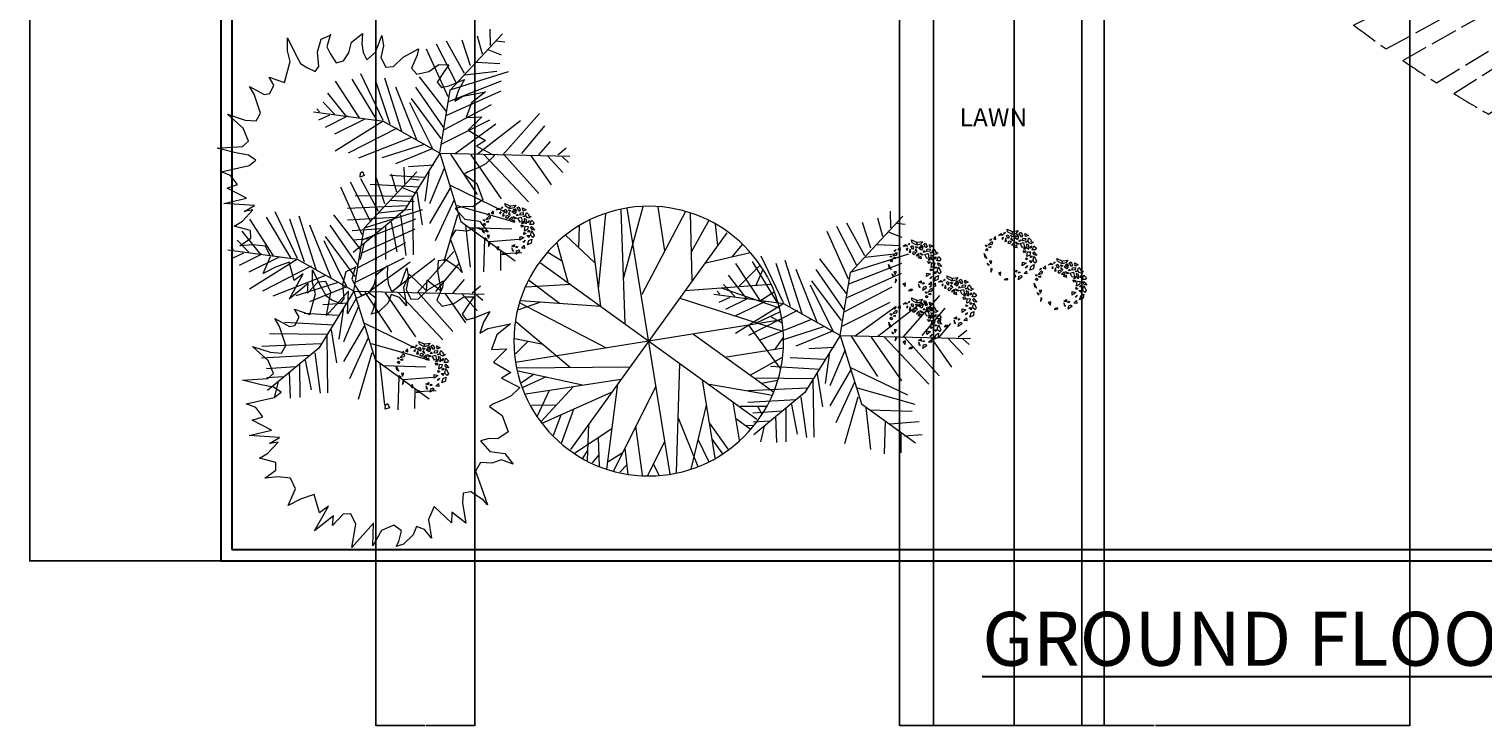
# Model space of a CAD drawing. Units: inches. Extents: x 2330 to 3943, y 1763 to 3461.
# Tile 1 of 40: x 2330 to 2977, y 1901 to 2211. Entities that reach past the tile are written whole.
import ezdxf

# ---------------------------------------------------------------- set-up
doc = ezdxf.new("R2010")
doc.units = ezdxf.units.IN
doc.linetypes.add('ACAD_ISO02W100', pattern=[15, 12, -3])
for name, color, linetype, lineweight in [('A-ANNO-DIMS', 2, 'Continuous', 18), ('A-ANNO-TEXT', 7, 'Continuous', 18), ('A-ANNO-TITL', 7, 'Continuous', 30), ('C-PROP', 7, 'Continuous', 30), ('L-PLNT', 94, 'Continuous', 13), ('L-PVMT-JOIN', 9, 'ACAD_ISO02W100', 13)]:
    doc.layers.add(name, color=color, linetype=linetype, lineweight=lineweight)
doc.styles.get("Standard").update_dxf_attribs({"font": 'arial.ttf'})
doc.dimstyles.get("Standard").update_dxf_attribs({"dimtxt": 0.18, "dimasz": 0.18, "dimexe": 0.18, "dimexo": 0.0625, "dimgap": 0.09, "dimtad": 0, "dimtih": 1, "dimtoh": 1, "dimdec": 4, "dimzin": 0, "dimdsep": 46, "dimtxsty": 'Standard', "dimcen": 0.09, "dimadec": 0, "dimazin": 0, "dimtfac": 1, "dimtdec": 4, "dimtofl": 0, "dimtmove": 0, "dimatfit": 3, "dimfxl": 1, "dimtolj": 1, "dimtzin": 0, "dimarcsym": 0})

# ---------------------------------------------------------------- blocks, each defined once
blk = doc.blocks.new('*U12')
for p, q in [((-8.737, 47.138), (-17.069, 52.711)), ((-10.186, 53.64), (-13.084, 55.962)), ((0, 0), (-10.5, 57)), ((-9.099, 51.782), (-6.563, 55.962)), ((-7.288, 39.707), (-21.778, 46.673)), ((-7.65, 43.423), (-2.578, 49.46)), ((-5.839, 35.992), (4.667, 48.067)), ((-5.114, 27.632), (10.463, 46.673)), ((-5.114, 28.097), (-24.676, 40.636)), ((-3.665, 19.273), (-27.574, 35.527)), ((-2.941, 16.486), (8.652, 37.85)), ((27, 9), (48, 36)), ((27.127, 9.056), (31.112, 35.992)), ((35.096, 32.741), (37.27, 22.524)), ((38.719, 34.134), (41.979, 28.561)), ((44.153, 36.456), (45.239, 32.741)), ((-48.585, 21.131), (-49.309, 29.026)), ((-43.513, 28.561), (-42.427, 15.558)), ((-38.442, 26.239), (-34.819, 7.663)), ((-35.544, 28.097), (-24.314, 3.947)), ((-1.129, 6.734), (9.014, 26.704)), ((10.101, 3.483), (17.708, 26.239)), ((16.259, 5.805), (23.142, 31.348)), ((22.055, 7.198), (27.489, 32.277)), ((31.836, 30.883), (32.561, 16.486)), ((43.791, 29.954), (51.036, 30.883)), ((-47.498, 19.737), (-55.83, 18.344)), ((-31.5, 4.5), (-52.5, 25.5)), ((-14.533, 2.09), (-30.834, 25.31)), ((-24.314, 23.917), (-2.941, 13.7)), ((3.942, 1.625), (11.187, 24.381)), ((36.183, 19.737), (48.137, 17.88)), ((40.53, 25.775), (48.862, 24.846)), ((-40.615, 13.7), (-55.105, 10.913)), ((-20.691, 13.7), (-1.129, 4.876)), ((33.285, 16.486), (48.862, 10.913)), ((0, 0), (27, 9)), ((24.229, 7.663), (46.688, 1.625)), ((29.662, 12.307), (48.137, 6.269)), ((-33.37, 6.269), (-52.207, 5.34)), ((-28.299, 3.483), (-47.86, -5.805)), ((-21.416, 3.018), (-38.079, -8.128)), ((0, 0), (-31.5, 4.5)), ((-15.982, 2.09), (-30.11, -9.521)), ((0, 0), (-22.5, -19.5)), ((-6.563, 1.161), (-21.416, -8.128)), ((0, 0), (18, -22.5)), ((6.478, 1.625), (26.04, -8.592)), ((11.187, 3.483), (30.749, -5.805)), ((18.07, 5.805), (35.096, -3.483)), ((-6.563, -5.805), (-19.967, -9.985)), ((-4.752, -3.483), (-3.665, -14.629)), ((2.493, -3.019), (-1.491, -20.202)), ((1.769, -2.555), (24.229, -9.521)), ((5.029, -6.27), (2.131, -25.775)), ((-15.257, -12.772), (-30.11, -12.772)), ((-13.446, -11.378), (-8.737, -32.741)), ((-9.461, -8.592), (-6.201, -23.453)), ((9.014, -11.378), (3.58, -35.992)), ((7.565, -9.056), (32.198, -14.629)), ((-17.431, -15.094), (-42.789, -18.809)), ((-20.691, -18.345), (-17.793, -44.352)), ((-17.069, -15.094), (-12.721, -40.172)), ((14.085, -16.951), (6.478, -40.172)), ((12.274, -15.094), (36.907, -18.809)), ((-24.314, -21.596), (-42.427, -22.06)), ((-26.849, -26.24), (-40.253, -25.775)), ((-22.5, -19.5), (-37.5, -45)), ((-25.038, -23.918), (-22.865, -45.281)), ((18.07, -22.524), (8.289, -45.745)), ((16.259, -19.738), (36.183, -22.989)), ((18, -22.5), (27, -52.5)), ((18.433, -22.524), (40.53, -29.026)), ((19.157, -25.311), (38.719, -33.206)), ((-28.299, -29.026), (-42.789, -31.348)), ((-29.023, -30.884), (-27.936, -43.887)), ((20.244, -30.419), (15.897, -44.816)), ((-30.834, -34.135), (-42.427, -35.528)), ((-32.646, -36.921), (-31.921, -44.352)), ((22.78, -37.85), (19.519, -48.532)), ((21.331, -32.741), (39.081, -40.636)), ((22.78, -38.314), (34.372, -44.816)), ((-34.457, -39.708), (-40.978, -42.494)), ((24.591, -43.423), (30.749, -47.603)), ((24.591, -45.745), (23.142, -50.854)), ((26.764, -49.925), (28.213, -50.854))]:
    blk.add_line(p, q)
blk = doc.blocks.new('*U13')
for points in [[(-5.78, 9.75), (-7.54, 9.23), (-8.01, 7.5), (-6.26, 8.45)], [(-5.78, 6.81), (-6.66, 6.21), (-6.52, 5.69)], [(-4.43, 11.05), (-5.18, 10.36), (-3.96, 9.49), (-2.07, 10.36)], [(-4.84, 8.63), (-3.83, 7.85), (-4.03, 8.97)], [(-2.88, 7.5), (-3.15, 6.64), (-2.27, 6.72)], [(-1.94, 9.49), (-2.48, 8.97), (-2.27, 8.54), (-1.8, 9.06)], [(-2, 11.66), (-1.6, 10.62), (-0.52, 10.1), (-0.18, 10.62), (-0.79, 10.96)], [(0.02, 9.06), (-1.33, 8.54), (-1.73, 7.16), (0.29, 7.76)], [(0.76, 7.16), (0.09, 6.46), (1.1, 5.95)], [(1.24, 12), (0.56, 11.31), (0.76, 10.01), (2.52, 11.05)], [(1.37, 8.54), (3.13, 8.8), (3.8, 7.85), (1.91, 7.76)], [(2.59, 9.93), (1.84, 9.75), (1.64, 9.23), (2.32, 9.41)], [(1.71, 6.29), (1.71, 7.07), (2.65, 7.5), (2.11, 6.9)], [(2.52, 6.81), (2.52, 5.86), (4.41, 5.17), (4.61, 6.72)], [(4.14, 11.14), (3.6, 10.01), (4, 9.23), (5.22, 8.71), (6.3, 9.41), (5.08, 10.19), (4.61, 10.01)], [(4.61, 8.28), (4.54, 7.76), (4.95, 7.59), (4.95, 8.28)], [(6.43, 7.94), (5.49, 7.68), (5.56, 6.21), (6.5, 6.64)], [(7.45, 9.32), (7.11, 7.94), (8.52, 7.94)], [(7.85, 6.81), (7.18, 6.21), (9, 5.51), (9.33, 6.38)], [(-11.32, 1.79), (-9.83, 2.31), (-9.63, 3.44), (-10.44, 3.52)], [(-8.21, 0.41), (-9.43, 0.32), (-9.83, 0.84)], [(-8.14, 6.03), (-9.36, 5.95), (-9.02, 4.73)], [(-8.21, 3.09), (-8.48, 2.31), (-7.87, 2.57)], [(-7, 1.79), (-7.94, 1.53), (-7.47, 0.49)], [(-4.57, 6.38), (-5.45, 4.47), (-3.89, 4.82)], [(3.53, 1.88), (2.86, 3.52), (3.8, 3.52)], [(4.41, 4.56), (4.27, 3.7), (5.49, 3.26)], [(4.27, 2.74), (5.29, 2.66), (4.41, 1.27)], [(5.83, 1.53), (5.02, 0.41), (5.49, -0.02), (6.5, 0.41)], [(5.49, 5.51), (5.42, 4.82), (6.16, 5.08)], [(7.51, 1.71), (6.91, 1.27), (6.23, 2.14)], [(8.12, 4.99), (7.11, 4.65), (6.5, 4.13), (7.38, 3.09), (8.12, 3.52), (7.65, 3.87)], [(8.12, 0.75), (7.51, 0.15), (8.93, -0.28), (9.13, 0.49)], [(8.19, 2.57), (7.92, 2.05), (8.66, 1.53)], [(8.73, 4.73), (8.19, 4.56), (8.39, 3.87), (8.59, 4.04)], [(10.28, 5.17), (9.2, 4.04), (9, 2.31), (10.48, 0.49), (11.76, 0.41), (10.35, 2.48), (9.33, 2.4), (10.28, 2.83)], [(-10.03, -2.71), (-10.64, -3.31), (-10.44, -4.44), (-9.9, -3.49)], [(-8.28, -5.73), (-6.79, -5.3), (-7, -6.51)], [(7.78, -0.8), (6.43, -1.5), (6.43, -0.72)], [(8.32, -1.75), (7.98, -2.53), (7.58, -2.1)], [(9.33, -5.13), (8.46, -6.25), (7.98, -5.22)], [(9.33, -1.75), (9.54, -3.74), (10.14, -2.53)], [(10.08, -0.63), (9.74, -1.32), (10.48, -0.89)], [(-4.84, -8.85), (-4.43, -9.45), (-5.99, -9.8)], [(-2.54, -10.06), (-3.02, -10.23), (-1.8, -10.67)], [(-2.34, -9.2), (-1.26, -8.5), (-0.99, -9.54)], [(0.22, -10.58), (0.83, -11.27), (2.59, -11.36)], [(4.07, -9.45), (3.53, -9.97), (4.07, -10.58), (4.61, -9.89)], [(5.29, -7.98), (4.61, -8.16), (5.02, -8.94)], [(6.03, -9.45), (5.42, -9.97), (6.16, -10.15)], [(6.1, -8.94), (6.16, -7.21), (6.91, -6.69), (7.24, -7.38)], [(8.05, -8.07), (8.59, -7.12), (7.92, -7.55)]]:
    blk.add_lwpolyline(points, close=True)
blk = doc.blocks.new('*U14')
for p, q in [((-12.5388, 54.9406), (-7.9613, 59.4546)), ((-12.3627, 32.1443), (-12.5388, 58.7776)), ((-5.3205, 59.6806), (16.5105, 16.7963)), ((2.426, 54.9406), (-1.4472, 59.9056)), ((0, 59.9996), (0, -60)), ((0.4894, 48.6208), (3.6584, 59.6806)), ((18.2711, 35.5298), (5.419, 59.6806)), ((9.8203, 51.5549), (12.8133, 58.5516)), ((-26.4472, 46.5894), (-26.2712, 53.8116)), ((-22.0458, 42.0753), (-16.5881, 57.6486)), ((-21.1656, 55.8436), (-0.0388, 45.0094)), ((19.6795, 19.5047), (16.3344, 57.6486)), ((17.0387, 51.1035), (23.2006, 55.1666)), ((17.7429, 43.6552), (25.4894, 54.2636)), ((-37.0107, 47.0408), (-35.25, 35.5298)), ((-32.6092, 50.4264), (-23.2782, 23.5674)), ((-31.2008, 51.1035), (-0.2149, 20.1818)), ((31.6513, 50.8778), (30.2429, 30.5643)), ((31.1232, 42.5267), (35.8767, 48.1693)), ((-43.8768, 36.4326), (-44.405, 40.2696)), ((42, 42), (-42, -42)), ((42, -42), (-42, 42)), ((-40.1797, 44.558), (-36.4825, 43.2038)), ((-49.8627, 32.8214), (-32.7853, 32.8214)), ((-45.8134, 38.2383), (-40.5318, 33.0471)), ((36.2288, 25.1474), (48.9049, 35.0784)), ((37.1091, 37.1098), (46.6161, 37.5612)), ((-53.2078, 27.4044), (-40.1797, 20.859)), ((23.3767, 23.3417), (53.3063, 27.4044)), ((-32.2571, 20.6333), (-59.1937, 9.348)), ((-56.0247, 20.859), (-20.8134, 20.859)), ((-54.7923, 24.4702), (-47.75, 21.0847)), ((54.3626, 25.3731), (20.9119, 0.3198)), ((-57.081, 17.9248), (-47.0458, 14.7649)), ((38.5175, 13.4107), (58.2359, 13.6364)), ((-59.7219, 2.8025), (-12.0106, 12.0565)), ((-58.6656, 12.7336), (-35.9543, 7.5424)), ((29.3626, -6.6771), (59.4682, 7.091)), ((-54.6162, -24.7335), (-20.2853, 0.0941)), ((-60, 0), (60, 0)), ((-59.7219, -4.8714), (-54.2641, -6.6771)), ((-45.2853, -0.1316), (-59.0177, -10.0627)), ((9.2922, -9.1598), (59.6443, -2.8401)), ((-58.4895, -12.3197), (-36.4825, -11.6426)), ((-10.074, -10.0627), (-2.5036, -59.7178)), ((26.3697, -18.4138), (58.9401, -9.8369)), ((-57.081, -18.4138), (-45.2853, -17.9624)), ((-52.6797, -18.188), (-55.4966, -22.0251)), ((-53.2078, -27.442), (-16.7641, -16.6081)), ((-47.2219, -19.3166), (-50.2148, -26.3135)), ((-14.8275, -15.0282), (-14.6515, -57.6865)), ((-0.0388, -19.0909), (25.8415, -53.8495)), ((18.6232, -18.6394), (26.7218, -53.3981)), ((18.7992, -18.6394), (57.3556, -17.2853)), ((38.1654, -18.188), (52.426, -29.0219)), ((-35.9543, -22.4765), (-44.0529, -40.5329)), ((-19.9331, -20.2194), (-28.5599, -52.721)), ((45.9119, -24.0564), (55.595, -22.2508)), ((-38.9472, -29.0219), (-51.4472, -30.6018)), ((-46.5177, -30.1504), (-49.5106, -33.536)), ((-14.6515, -32.1818), (-3.912, -59.4922)), ((30.419, -30.1504), (32.3556, -50.0125)), ((31.4753, -31.279), (49.6091, -33.3103)), ((-32.4331, -32.4075), (-48.1021, -35.5674)), ((-43.7008, -34.6645), (-46.6937, -37.373)), ((-24.6867, -37.8244), (-38.7712, -45.7241)), ((-14.6515, -36.2445), (-27.6797, -52.9467)), ((-6.2008, -36.2445), (17.919, -57.0094)), ((22.8485, -36.4702), (35.3485, -48.4326)), ((41.5105, -32.6332), (46.088, -38.0501)), ((-26.2712, -43.9185), (-34.7219, -48.6583)), ((24.7852, -44.8213), (23.0246, -54.978)), ((-14.6515, -47.3041), (-25.0388, -54.3009)), ((-21.5177, -45.4984), (-19.9331, -56.1065)), ((-8.4895, -47.5298), (-11.4825, -58.5893)), ((5.9471, -46.6269), (10.5246, -58.5893)), ((-6.3768, -52.721), (-9.3698, -58.815)), ((8.4119, -53.1724), (3.8344, -59.4922))]:
    blk.add_line(p, q)
blk.add_circle((0, 0), 60)
blk = doc.blocks.new('*U15')
for points in [[(0, 60.64), (-3.051, 56.238), (-4.196, 52.815), (-5.34, 47.925), (-6.103, 45.969), (-11.062, 50.859), (-18.691, 52.326), (-20.98, 47.436), (-20.217, 43.524), (-20.598, 39.611), (-25.939, 43.035), (-27.846, 49.392), (-33.186, 52.326), (-30.516, 47.436), (-31.279, 43.035), (-30.135, 38.144), (-33.568, 35.21), (-40.815, 36.677), (-49.208, 38.144), (-46.919, 36.677), (-42.341, 31.787), (-42.341, 28.364), (-46.537, 27.386), (-55.692, 27.386), (-49.97, 22.006), (-54.548, 21.028), (-46.156, 14.671), (-51.496, 11.248), (-59.888, 11.248), (-55.692, 8.803), (-53.785, 5.38), (-57.218, 3.423), (-60.651, -1.467), (-61.033, -4.89), (-59.125, -3.423), (-54.548, -1.467), (-51.496, -4.401), (-53.022, -10.269), (-59.125, -15.16), (-49.208, -13.204), (-58.362, -24.451), (-48.445, -21.028), (-43.486, -22.495), (-43.104, -25.918), (-47.3, -31.298), (-43.104, -30.32), (-48.445, -39.611), (-38.527, -31.787), (-40.815, -36.188), (-32.423, -37.166), (-33.568, -43.523), (-35.475, -49.392), (-28.609, -44.99), (-23.65, -46.457), (-22.124, -51.837), (-21.743, -57.705), (-19.073, -52.326), (-15.639, -51.837), (-12.588, -58.683), (-11.062, -54.771), (-6.866, -49.392), (-6.866, -53.304), (-4.959, -48.414), (-1.907, -61.617), (-1.144, -51.348), (4.578, -59.172), (5.341, -54.282), (9.918, -56.727), (12.207, -60.639), (12.97, -47.925), (14.877, -44.501), (17.547, -47.436), (19.455, -52.815), (22.888, -60.639), (21.743, -49.392), (23.65, -46.457), (29.754, -47.925), (35.094, -52.326), (37.001, -53.793), (33.187, -46.457), (32.042, -41.567), (35.094, -39.122), (43.868, -40.589), (47.682, -42.056), (43.105, -36.188), (43.105, -33.743), (46.538, -31.298), (50.352, -32.765), (46.919, -26.407), (55.693, -22.495), (60.652, -22.984), (66.374, -22.006), (59.889, -20.05), (54.167, -18.094), (51.878, -15.649), (49.589, -12.225), (51.497, -10.269), (57.981, -9.78), (63.322, -7.335), (64.466, -2.934)], [(64.848, -2.934), (59.507, -5.379), (56.456, -4.401), (51.878, -2.445), (52.26, 0.978), (55.311, 3.912), (59.889, 5.869), (62.94, 11.248), (58.363, 10.27), (54.548, 10.27), (51.115, 11.248), (53.785, 15.649), (57.981, 18.094), (60.652, 19.561), (56.074, 19.561), (51.115, 17.605), (46.538, 19.072), (46.156, 22.496), (49.589, 27.386), (52.26, 34.721), (49.589, 33.743), (44.249, 30.32), (41.197, 32.276), (41.579, 37.655), (43.868, 42.546), (43.105, 46.947), (40.053, 44.013), (36.238, 40.589), (33.568, 42.057), (33.95, 45.969), (35.476, 52.815), (31.28, 49.392), (26.702, 46.947), (28.228, 50.859), (28.609, 61.129), (24.795, 54.282), (18.692, 50.859), (17.929, 57.706), (12.97, 50.859), (7.248, 57.706), (5.341, 53.304), (0, 60.64)]]:
    blk.add_lwpolyline(points)
blk.add_lwpolyline([(0.382, 1.956), (0, 0), (1.907, 0.489), (2.289, 1.467)], close=True)
blk = doc.blocks.new('PAVER-RADIAL')
for p, q in [((0, 15.76), (109.7, 19.29)), ((8.7, 0), (118.23, 7.05))]:
    blk.add_line(p, q)
for radius, start, end in [(559.83, 207.9852, 209.8274), (463.83, 213.96986, 215.81207)]:
    blk.add_arc((494.37, 278.45), radius, start, end)
blk = doc.blocks.new('*D60')
at = {"layer": 'A-ANNO-DIMS', "color": 0, "lineweight": -2, "transparency": 16777216}
for p, q in [((2415.6, 3210.65), (2330.5, 3210.65)), ((2330.68, 3210.47), (2330.68, 2592.83)), ((2330.68, 1974.83), (2330.68, 2592.47)), ((2415.6, 1974.65), (2330.5, 1974.65))]:
    blk.add_line(p, q, dxfattribs=at)
at = {"layer": 'A-ANNO-DIMS', "color": 0, "transparency": 16777216}
for points in [[(2330.65, 3210.47), (2330.71, 3210.47), (2330.68, 3210.65)], [(2330.65, 1974.83), (2330.71, 1974.83), (2330.68, 1974.65)]]:
    blk.add_solid(points, dxfattribs=at)
at = {"layer": 'Defpoints', "color": 0, "transparency": 16777216}
for p in [(2330.68, 3210.65), (2415.66, 3210.65), (2415.66, 1974.65)]:
    blk.add_point(p, dxfattribs=at)
at = {"layer": 'A-ANNO-DIMS', "color": 0, "transparency": 16777216, "insert": (2330.68, 2592.65), "char_height": 0.18, "attachment_point": 5}
blk.add_mtext('\\A1;1236', dxfattribs=at)
blk = doc.blocks.new('*D70')
at = {"layer": 'A-ANNO-DIMS', "color": 0, "lineweight": -2, "transparency": 16777216}
for p, q in [((2732.66, 2606.59), (2732.66, 1901.2)), ((2768.66, 2606.59), (2768.66, 1901.2)), ((2732.84, 1901.38), (2750.44, 1901.38)), ((2768.48, 1901.38), (2750.88, 1901.38))]:
    blk.add_line(p, q, dxfattribs=at)
at = {"layer": 'A-ANNO-DIMS', "color": 0, "transparency": 16777216}
for points in [[(2732.84, 1901.41), (2732.84, 1901.35), (2732.66, 1901.38)], [(2768.48, 1901.41), (2768.48, 1901.35), (2768.66, 1901.38)]]:
    blk.add_solid(points, dxfattribs=at)
at = {"layer": 'Defpoints', "color": 0, "transparency": 16777216}
for p in [(2732.66, 2606.65), (2768.66, 2606.65), (2768.66, 1901.38)]:
    blk.add_point(p, dxfattribs=at)
at = {"layer": 'A-ANNO-DIMS', "color": 0, "transparency": 16777216, "insert": (2750.66, 1901.38), "char_height": 0.18, "attachment_point": 5}
blk.add_mtext('\\A1;36', dxfattribs=at)
blk = doc.blocks.new('*D73')
at = {"layer": 'A-ANNO-DIMS', "color": 0, "lineweight": -2, "transparency": 16777216}
for p, q in [((2798.66, 2676.59), (2798.66, 1901.2)), ((2808.66, 2676.59), (2808.66, 1901.2)), ((2798.84, 1901.38), (2803.45, 1901.38)), ((2808.48, 1901.38), (2803.87, 1901.38))]:
    blk.add_line(p, q, dxfattribs=at)
at = {"layer": 'A-ANNO-DIMS', "color": 0, "transparency": 16777216}
for points in [[(2798.84, 1901.41), (2798.84, 1901.35), (2798.66, 1901.38)], [(2808.48, 1901.41), (2808.48, 1901.35), (2808.66, 1901.38)]]:
    blk.add_solid(points, dxfattribs=at)
at = {"layer": 'Defpoints', "color": 0, "transparency": 16777216}
for p in [(2798.66, 2676.65), (2808.66, 2676.65), (2808.66, 1901.38)]:
    blk.add_point(p, dxfattribs=at)
at = {"layer": 'A-ANNO-DIMS', "color": 0, "transparency": 16777216, "insert": (2803.66, 1901.38), "char_height": 0.18, "attachment_point": 5}
blk.add_mtext('\\A1;10', dxfattribs=at)
blk = doc.blocks.new('*D77')
at = {"layer": 'A-ANNO-DIMS', "color": 0, "lineweight": -2, "transparency": 16777216}
for p, q in [((2717.66, 2412.59), (2717.66, 1901.2)), ((2944.66, 2412.59), (2944.66, 1901.2)), ((2717.84, 1901.38), (2830.87, 1901.38)), ((2944.48, 1901.38), (2831.45, 1901.38))]:
    blk.add_line(p, q, dxfattribs=at)
at = {"layer": 'A-ANNO-DIMS', "color": 0, "transparency": 16777216}
for points in [[(2717.84, 1901.41), (2717.84, 1901.35), (2717.66, 1901.38)], [(2944.48, 1901.41), (2944.48, 1901.35), (2944.66, 1901.38)]]:
    blk.add_solid(points, dxfattribs=at)
at = {"layer": 'Defpoints', "color": 0, "transparency": 16777216}
for p in [(2717.66, 2412.65), (2944.66, 2412.65), (2944.66, 1901.38)]:
    blk.add_point(p, dxfattribs=at)
at = {"layer": 'A-ANNO-DIMS', "color": 0, "transparency": 16777216, "insert": (2831.16, 1901.38), "char_height": 0.18, "attachment_point": 5}
blk.add_mtext('\\A1;227', dxfattribs=at)
blk = doc.blocks.new('*D90')
at = {"layer": 'A-ANNO-DIMS', "color": 0, "lineweight": -2, "transparency": 16777216}
for p, q in [((2484.66, 3153.59), (2484.66, 1901.2)), ((2528.66, 3153.59), (2528.66, 1901.2)), ((2484.84, 1901.38), (2506.44, 1901.38)), ((2528.48, 1901.38), (2506.88, 1901.38))]:
    blk.add_line(p, q, dxfattribs=at)
at = {"layer": 'A-ANNO-DIMS', "color": 0, "transparency": 16777216}
for points in [[(2484.84, 1901.41), (2484.84, 1901.35), (2484.66, 1901.38)], [(2528.48, 1901.41), (2528.48, 1901.35), (2528.66, 1901.38)]]:
    blk.add_solid(points, dxfattribs=at)
at = {"layer": 'Defpoints', "color": 0, "transparency": 16777216}
for p in [(2484.66, 3153.65), (2528.66, 3153.65), (2528.66, 1901.38)]:
    blk.add_point(p, dxfattribs=at)
at = {"layer": 'A-ANNO-DIMS', "color": 0, "transparency": 16777216, "insert": (2506.66, 1901.38), "char_height": 0.18, "attachment_point": 5}
blk.add_mtext('\\A1;44', dxfattribs=at)

msp = doc.modelspace()

# ---------------------------------------------------------------- linework, layer by layer
at = {"layer": 'C-PROP'}
for p, q in [((2415.6605, 3210.6524), (2415.6605, 1974.6524)), ((2420.6605, 3205.6524), (2420.6605, 1979.6524)), ((2420.6605, 1979.6524), (3439.5159, 1979.6524)), ((2415.6605, 1974.6524), (3439.5159, 1974.6524))]:
    msp.add_line(p, q, dxfattribs=at)

# ---------------------------------------------------------------- block references
at = {"layer": 'L-PLNT', "xscale": -1, "rotation": 279.1543537978463}
for name, p in [('*U15', (2477.6333, 2145.4094)), ('*U12', (2513.0823, 2155.9909)), ('*U12', (2474.9288, 2094.5909)), ('*U14', (2606.0658, 2072.4199)), ('*U13', (2543.4518, 2121.9898)), ('*U12', (2691.1949, 2074.8995)), ('*U13', (2766.897, 2110.6413)), ('*U15', (2488.8298, 2042.1191)), ('*U13', (2724.3981, 2105.8115)), ('*U13', (2789.0641, 2097.5148)), ('*U13', (2740.1466, 2089.8188)), ('*U13', (2724.4242, 2080.0707)), ('*U13', (2505.2983, 2060.5897))]:
    msp.add_blockref(name, p, dxfattribs=at)
at = {"layer": 'L-PVMT-JOIN'}
for p, rotation in [((2926.2218, 2198.7785), 24.86978119553056), ((2948.81, 2183.3363), 27.63309021683611), ((2972.1164, 2169.001), 30.39639923898183)]:
    msp.add_blockref('PAVER-RADIAL', p, dxfattribs=dict(at, rotation=rotation))

# ---------------------------------------------------------------- texts
at = {"layer": 'A-ANNO-TEXT', "insert": (2744.3558, 2175.9689), "char_height": 8, "attachment_point": 1}
msp.add_mtext_dynamic_manual_height_columns('LAWN', width=151.739694, gutter_width=12.5, heights=[0], dxfattribs=at)
at = {"layer": 'A-ANNO-TITL', "insert": (2754.4138, 1951.9773), "char_height": 24, "attachment_point": 1}
msp.add_mtext_dynamic_manual_height_columns('{\\LGROUND FLOOR PLAN}', width=457.144969, gutter_width=12.5, heights=[0], dxfattribs=at)

# ---------------------------------------------------------------- dimensions: what is measured, and where the dimension line sits
at = {"layer": 'A-ANNO-DIMS'}
dim = msp.add_linear_dim(base=(2330.6824, 3210.6524), p1=(2415.6605, 1974.6524), p2=(2415.6605, 3210.6524), angle=90, dimstyle='Standard', override={"dimdec": 0, "dimlfac": 1, "dimrnd": 0, "dimzin": 0, "dimdsep": 46, "dimlunit": 2}, dxfattribs=at)
dim.commit()
dim.dimension.update_dxf_attribs({"geometry": '*D60', "text_midpoint": (2330.6824, 2592.6524)})
for base, p1, p2, picture, middle in [((2528.6605, 1901.3774), (2484.6605, 3153.6524), (2528.6605, 3153.6524), '*D90', (2506.6605, 1901.3774)), ((2808.6605, 1901.3774), (2798.6605, 2676.6524), (2808.6605, 2676.6524), '*D73', (2803.6605, 1901.3774)), ((2768.6605, 1901.3774), (2732.6605, 2606.6524), (2768.6605, 2606.6524), '*D70', (2750.6605, 1901.3774)), ((2944.6605, 1901.3774), (2717.6605, 2412.6524), (2944.6605, 2412.6524), '*D77', (2831.1605, 1901.3774))]:
    dim = msp.add_linear_dim(base=base, p1=p1, p2=p2, dimstyle='Standard', override={"dimdec": 0, "dimlfac": 1, "dimrnd": 0, "dimzin": 0, "dimdsep": 46, "dimlunit": 2}, dxfattribs=at)
    dim.commit()
    dim.dimension.update_dxf_attribs({"geometry": picture, "text_midpoint": middle})

doc.saveas('drawing.dxf')
